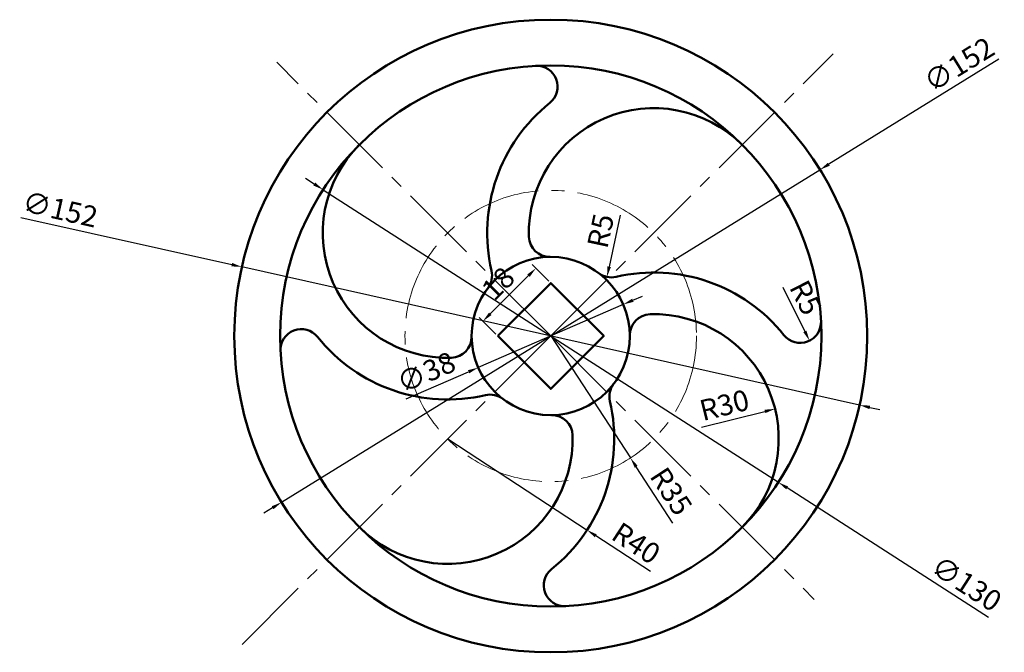
# Model space of a CAD drawing. Units: millimetres. Extents: x 3285 to 3522, y 1620 to 1772.
import ezdxf

# ---------------------------------------------------------------- set-up
doc = ezdxf.new("R2010")
doc.units = ezdxf.units.MM
doc.linetypes.add('CENTER2', pattern=[28.575, 19.05, -3.175, 3.175, -3.175])
for name, color, linetype, lineweight in [('M-CNTR', 50, 'CENTER2', 18), ('M-DIMS', 2, 'Continuous', 25), ('M-OUTL', 7, 'Continuous', 50)]:
    doc.layers.add(name, color=color, linetype=linetype, lineweight=lineweight)
doc.styles.get("Standard").update_dxf_attribs({"font": 'arial.ttf'})
doc.dimstyles.new('ISO-25', dxfattribs={"dimtxt": 5, "dimasz": 2.5, "dimexe": 1.25, "dimexo": 0.625, "dimtad": 1, "dimtxsty": 'Standard', "dimcen": 2.5, "dimadec": 0, "dimazin": 0, "dimtfac": 1, "dimtmove": 0, "dimatfit": 3, "dimfxl": 1, "dimarcsym": 0})

# ---------------------------------------------------------------- blocks, each defined once
blk = doc.blocks.new('*D1')
at = {"layer": 'Defpoints', "color": 0, "transparency": 16777216}
for p in [(3409.32, 1712.39), (3412.88, 1708.83), (3400.15, 1696.11)]:
    blk.add_point(p, dxfattribs=at)
at = {"layer": 'M-DIMS', "color": 0, "lineweight": -2, "transparency": 16777216}
for p, q in [((3412.44, 1709.28), (3408.43, 1713.28)), ((3398.36, 1701.43), (3407.55, 1710.63)), ((3399.71, 1696.55), (3395.71, 1700.55))]:
    blk.add_line(p, q, dxfattribs=at)
at = {"layer": 'M-DIMS', "color": 0, "transparency": 16777216}
for points in [[(3407.26, 1710.92), (3407.85, 1710.33), (3409.32, 1712.39)], [(3398.06, 1701.73), (3398.65, 1701.14), (3396.59, 1699.67)]]:
    blk.add_solid(points, dxfattribs=at)
at = {"layer": 'M-DIMS', "color": 0, "transparency": 16777216, "insert": (3400.71, 1708.28), "char_height": 5, "attachment_point": 5, "rotation": 45}
blk.add_mtext('18', dxfattribs=at)
blk = doc.blocks.new('*D2')
at = {"layer": 'Defpoints', "color": 0, "transparency": 16777216}
for p in [(3427.44, 1715.19), (3426.39, 1710.3)]:
    blk.add_point(p, dxfattribs=at)
at = {"layer": 'M-DIMS', "color": 0, "lineweight": -2, "transparency": 16777216}
blk.add_line((3429.57, 1725.12), (3426.91, 1712.74), dxfattribs=at)
at = {"layer": 'M-DIMS', "color": 0, "transparency": 16777216}
blk.add_solid([(3426.5, 1712.83), (3427.32, 1712.66), (3426.39, 1710.3)], dxfattribs=at)
at = {"layer": 'M-DIMS', "color": 0, "transparency": 16777216, "insert": (3425.49, 1721.22), "char_height": 5, "attachment_point": 5, "rotation": 77.8732}
blk.add_mtext('R5', dxfattribs=at)
blk = doc.blocks.new('*D3')
at = {"layer": 'Defpoints', "color": 0, "transparency": 16777216}
for p in [(3472.79, 1699.44), (3475.03, 1694.98)]:
    blk.add_point(p, dxfattribs=at)
at = {"layer": 'M-DIMS', "color": 0, "lineweight": -2, "transparency": 16777216}
blk.add_line((3468.59, 1707.8), (3473.91, 1697.21), dxfattribs=at)
at = {"layer": 'M-DIMS', "color": 0, "transparency": 16777216}
blk.add_solid([(3474.28, 1697.4), (3473.54, 1697.02), (3475.03, 1694.98)], dxfattribs=at)
at = {"layer": 'M-DIMS', "color": 0, "transparency": 16777216, "insert": (3473.52, 1705.04), "char_height": 5, "attachment_point": 5, "rotation": 296.6466}
blk.add_mtext('R5', dxfattribs=at)
blk = doc.blocks.new('*D4')
at = {"layer": 'Defpoints', "color": 0, "transparency": 16777216}
for p in [(3466.74, 1678.59), (3437.63, 1671.36)]:
    blk.add_point(p, dxfattribs=at)
at = {"layer": 'M-DIMS', "color": 0, "lineweight": -2, "transparency": 16777216}
blk.add_line((3449.1, 1674.21), (3464.32, 1677.99), dxfattribs=at)
at = {"layer": 'M-DIMS', "color": 0, "transparency": 16777216}
blk.add_solid([(3464.22, 1678.39), (3464.42, 1677.58), (3466.74, 1678.59)], dxfattribs=at)
at = {"layer": 'M-DIMS', "color": 0, "transparency": 16777216, "insert": (3454.73, 1678.88), "char_height": 5, "attachment_point": 5, "rotation": 13.9549}
blk.add_mtext('R30', dxfattribs=at)
blk = doc.blocks.new('*D5')
at = {"layer": 'Defpoints', "color": 0, "transparency": 16777216}
for p in [(3412.88, 1696.11), (3432.02, 1666.81)]:
    blk.add_point(p, dxfattribs=at)
at = {"layer": 'M-DIMS', "color": 0, "lineweight": -2, "transparency": 16777216}
for p, q in [((3412.88, 1696.11), (3432.02, 1666.81)), ((3442.24, 1651.17), (3433.39, 1664.71))]:
    blk.add_line(p, q, dxfattribs=at)
at = {"layer": 'M-DIMS', "color": 0, "transparency": 16777216}
blk.add_solid([(3433.74, 1664.94), (3433.04, 1664.48), (3432.02, 1666.81)], dxfattribs=at)
at = {"layer": 'M-DIMS', "color": 0, "transparency": 16777216, "insert": (3441.28, 1658.45), "char_height": 5, "attachment_point": 5, "rotation": 303.1592}
blk.add_mtext('R35', dxfattribs=at)
blk = doc.blocks.new('*D6')
at = {"layer": 'Defpoints', "color": 0, "transparency": 16777216}
for p in [(3388.13, 1671.36), (3421.61, 1649.47)]:
    blk.add_point(p, dxfattribs=at)
at = {"layer": 'M-DIMS', "color": 0, "lineweight": -2, "transparency": 16777216}
for p, q in [((3388.13, 1671.36), (3421.61, 1649.47)), ((3436.83, 1639.52), (3423.7, 1648.1))]:
    blk.add_line(p, q, dxfattribs=at)
at = {"layer": 'M-DIMS', "color": 0, "transparency": 16777216}
blk.add_solid([(3423.93, 1648.45), (3423.47, 1647.75), (3421.61, 1649.47)], dxfattribs=at)
at = {"layer": 'M-DIMS', "color": 0, "transparency": 16777216, "insert": (3433.05, 1645.78), "char_height": 5, "attachment_point": 5, "rotation": 326.8209}
blk.add_mtext('R40', dxfattribs=at)
blk = doc.blocks.new('*D7')
at = {"layer": 'Defpoints', "color": 0, "transparency": 16777216}
for p in [(3477.53, 1736.05), (3348.23, 1656.16)]:
    blk.add_point(p, dxfattribs=at)
at = {"layer": 'M-DIMS', "color": 0, "lineweight": -2, "transparency": 16777216}
for p, q in [((3520.52, 1762.62), (3479.66, 1737.37)), ((3348.23, 1656.16), (3477.53, 1736.05)), ((3346.1, 1654.84), (3343.97, 1653.53))]:
    blk.add_line(p, q, dxfattribs=at)
at = {"layer": 'M-DIMS', "color": 0, "transparency": 16777216}
for points in [[(3479.44, 1737.72), (3479.88, 1737.01), (3477.53, 1736.05)], [(3345.88, 1655.2), (3346.32, 1654.49), (3348.23, 1656.16)]]:
    blk.add_solid(points, dxfattribs=at)
at = {"layer": 'M-DIMS', "color": 0, "transparency": 16777216, "insert": (3511.25, 1760.79), "char_height": 5, "attachment_point": 5, "rotation": 31.7118}
blk.add_mtext('∅152', dxfattribs=at)
blk = doc.blocks.new('*D8')
at = {"layer": 'Defpoints', "color": 0, "transparency": 16777216}
for p in [(3358.21, 1731.26), (3467.55, 1660.95)]:
    blk.add_point(p, dxfattribs=at)
at = {"layer": 'M-DIMS', "color": 0, "lineweight": -2, "transparency": 16777216}
for p, q in [((3356.1, 1732.61), (3354, 1733.97)), ((3358.21, 1731.26), (3467.55, 1660.95)), ((3518.04, 1628.48), (3469.65, 1659.6))]:
    blk.add_line(p, q, dxfattribs=at)
at = {"layer": 'M-DIMS', "color": 0, "transparency": 16777216}
for points in [[(3356.33, 1732.97), (3355.88, 1732.26), (3358.21, 1731.26)], [(3469.88, 1659.95), (3469.43, 1659.25), (3467.55, 1660.95)]]:
    blk.add_solid(points, dxfattribs=at)
at = {"layer": 'M-DIMS', "color": 0, "transparency": 16777216, "insert": (3512.38, 1636.06), "char_height": 5, "attachment_point": 5, "rotation": 327.2567}
blk.add_mtext('∅130', dxfattribs=at)
blk = doc.blocks.new('*D9')
at = {"layer": 'Defpoints', "color": 0, "transparency": 16777216}
for p in [(3430.3, 1703.69), (3395.46, 1688.52)]:
    blk.add_point(p, dxfattribs=at)
at = {"layer": 'M-DIMS', "color": 0, "lineweight": -2, "transparency": 16777216}
for p, q in [((3432.59, 1704.69), (3434.88, 1705.69)), ((3430.3, 1703.69), (3395.46, 1688.52)), ((3378.17, 1680.99), (3393.17, 1687.52))]:
    blk.add_line(p, q, dxfattribs=at)
at = {"layer": 'M-DIMS', "color": 0, "transparency": 16777216}
for points in [[(3432.42, 1705.07), (3432.76, 1704.31), (3430.3, 1703.69)], [(3393, 1687.9), (3393.33, 1687.14), (3395.46, 1688.52)]]:
    blk.add_solid(points, dxfattribs=at)
at = {"layer": 'M-DIMS', "color": 0, "transparency": 16777216, "insert": (3383.2, 1686.8), "char_height": 5, "attachment_point": 5, "rotation": 23.5321}
blk.add_mtext('∅38', dxfattribs=at)
blk = doc.blocks.new('ROTOR-BLADE')
for points in [[(53.38, 49.58, -0.730343), (44.48, 46.18, 0.288968), (4.16, 60.17, -0.223658), (0, 61.07)], [(34.44, 0, 0.679083), (12.33, 51.2, 0.408367), (7.48, 46.15)]]:
    blk.add_lwpolyline(points, format="xyb")
blk = doc.blocks.new('*D11')
at = {"layer": 'Defpoints', "color": 0, "transparency": 16777216}
for p in [(3338.71, 1712.7), (3487.04, 1679.51)]:
    blk.add_point(p, dxfattribs=at)
at = {"layer": 'M-DIMS', "color": 0, "lineweight": -2, "transparency": 16777216}
for p, q in [((3285.59, 1724.59), (3336.27, 1713.25)), ((3487.04, 1679.51), (3338.71, 1712.7)), ((3489.48, 1678.96), (3491.92, 1678.42))]:
    blk.add_line(p, q, dxfattribs=at)
at = {"layer": 'M-DIMS', "color": 0, "transparency": 16777216}
for points in [[(3336.37, 1713.66), (3336.18, 1712.84), (3338.71, 1712.7)], [(3489.58, 1679.37), (3489.39, 1678.55), (3487.04, 1679.51)]]:
    blk.add_solid(points, dxfattribs=at)
at = {"layer": 'M-DIMS', "color": 0, "transparency": 16777216, "insert": (3294.94, 1725.9), "char_height": 5, "attachment_point": 5, "rotation": 347.3852}
blk.add_mtext('∅152', dxfattribs=at)

msp = doc.modelspace()

# ---------------------------------------------------------------- linework, layer by layer
at = {"layer": 'M-CNTR'}
for q in [(3347.066, 1761.918), (3480.673, 1763.9), (3338.069, 1621.296), (3476.159, 1632.825)]:
    msp.add_line((3412.879, 1696.106), q, dxfattribs=at)
msp.add_circle((3412.879, 1696.106), 35, dxfattribs=at)
at = {"layer": 'M-OUTL'}
msp.add_lwpolyline([(3400.151, 1696.106), (3412.879, 1683.378), (3425.607, 1696.106), (3412.879, 1708.834)], close=True, dxfattribs=at)
for radius in [76, 65, 19]:
    msp.add_circle((3412.879, 1696.106), radius, dxfattribs=at)
msp.add_arc((3388.13, 1671.357), 40, 73.35764, 73.95502, dxfattribs=at)

# ---------------------------------------------------------------- block references
for p, rotation in [((3458.841, 1707.629), 89.99999999999793), ((3401.355, 1742.067), 180), ((3366.918, 1684.582), 269.9999999999956)]:
    msp.add_blockref('ROTOR-BLADE', p, dxfattribs=dict(at, rotation=rotation))
msp.add_blockref('ROTOR-BLADE', (3424.403, 1650.144), dxfattribs=at)

# ---------------------------------------------------------------- dimensions: what is measured, and where the dimension line sits
at = {"layer": 'M-DIMS'}
for p1, p2, override, picture, middle in [((3348.226, 1656.156), (3477.533, 1736.055), {"dimclrd": 0, "dimclre": 0, "dimclrt": 0}, '*D7', (3512.996, 1757.967)), ((3358.208, 1731.263), (3467.551, 1660.949), {"dimclrd": 0, "dimclre": 0, "dimclrt": 0}, '*D8', (3510.589, 1633.273)), ((3487.045, 1679.508), (3338.714, 1712.704), {"dimdec": 0, "dimlfac": 1, "dimrnd": 0, "dimzin": 0, "dimdsep": 46, "dimlunit": 2}, '*D11', (3294.215, 1722.662))]:
    dim = msp.add_diameter_dim_2p(p1=p1, p2=p2, dimstyle='ISO-25', override=override, dxfattribs=at)
    dim.commit()
    dim.dimension.update_dxf_attribs({"geometry": picture, "text_midpoint": middle, "dimtype": 163})
for center, mpoint, picture, middle in [((3427.436, 1715.187), (3426.385, 1710.299), '*D2', (3428.588, 1720.55)), ((3472.786, 1699.444), (3475.029, 1694.975), '*D3', (3470.69, 1703.623)), ((3412.879, 1696.106), (3432.023, 1666.805), '*D5', (3438.62, 1656.709)), ((3437.628, 1671.357), (3466.743, 1678.592), '*D4', (3455.494, 1675.797))]:
    dim = msp.add_radius_dim(center=center, mpoint=mpoint, dimstyle='ISO-25', override={"dimclrd": 0, "dimclre": 0, "dimclrt": 0}, dxfattribs=at)
    dim.commit()
    dim.dimension.update_dxf_attribs({"geometry": picture, "text_midpoint": middle, "dimtype": 164})
dim = msp.add_aligned_dim(p1=(3400.151, 1696.106), p2=(3412.879, 1708.834), distance=5.036, dimstyle='ISO-25', override={"dimclrd": 0, "dimclre": 0, "dimclrt": 0}, dxfattribs=at)
dim.commit()
dim.dimension.update_dxf_attribs({"geometry": '*D1', "text_midpoint": (3400.707, 1708.277)})
dim = msp.add_diameter_dim_2p(p1=(3430.299, 1703.692), p2=(3395.459, 1688.52), dimstyle='ISO-25', override={"dimclrd": 0, "dimclre": 0, "dimclrt": 0}, dxfattribs=at)
dim.commit()
dim.dimension.update_dxf_attribs({"geometry": '*D9', "text_midpoint": (3383.196, 1686.798)})
dim = msp.add_radius_dim(center=(3388.13, 1671.357), mpoint=(3421.609, 1649.467), dimstyle='ISO-25', override={"dimclrd": 0, "dimclre": 0, "dimclrt": 0}, dxfattribs=at)
dim.commit()
dim.dimension.update_dxf_attribs({"geometry": '*D6', "text_midpoint": (3433.049, 1645.783)})

doc.saveas('drawing.dxf')
